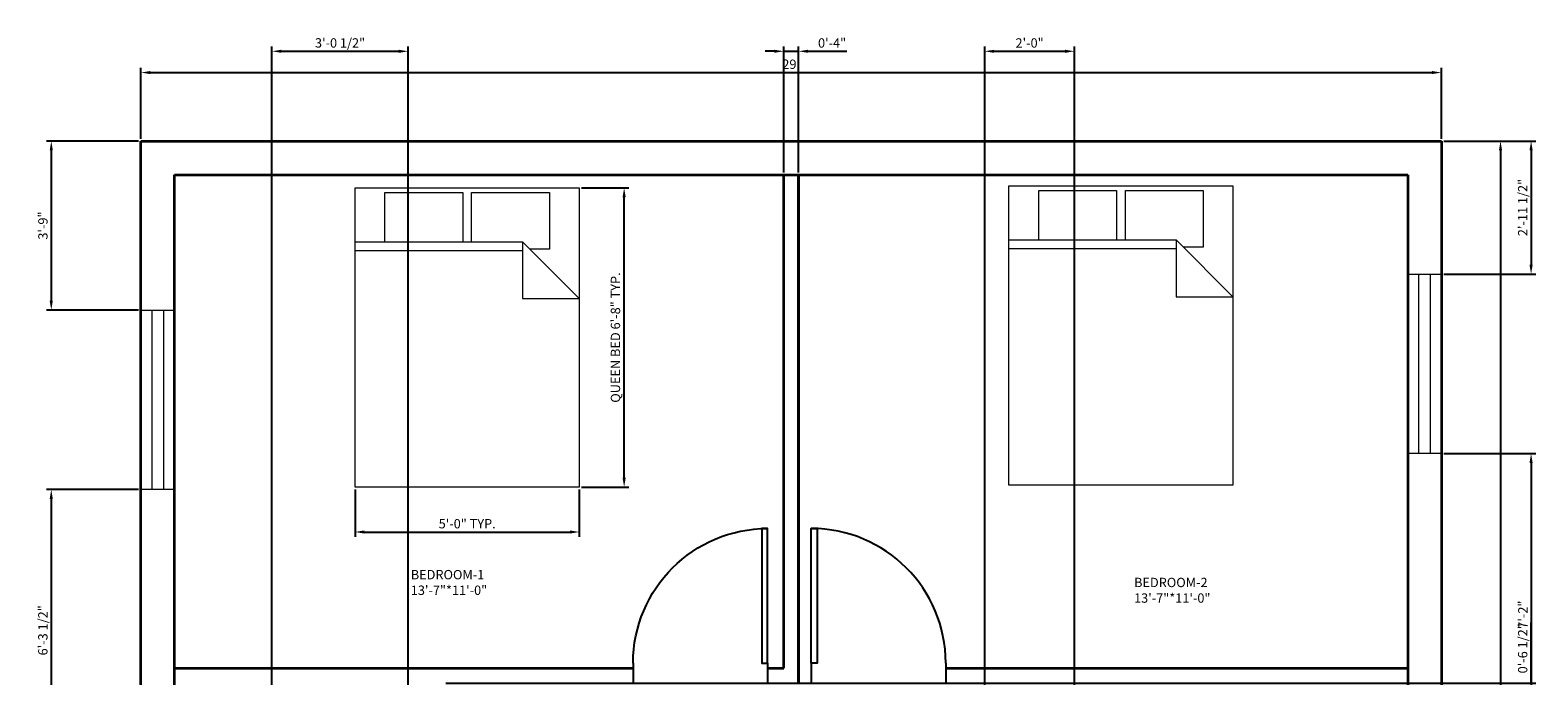
# Model space of a CAD drawing. Units: inches. Extents: x 2655 to 3059, y 1617 to 2098.
# Tile 3 of 3: x 2655 to 3059, y 1926 to 2098. Entities that reach past the tile are written whole.
import ezdxf

# ---------------------------------------------------------------- set-up
doc = ezdxf.new("R2010")
doc.units = ezdxf.units.IN
for name, color, linetype, lineweight in [('A-ANNO-DIMS', 2, 'Continuous', 18), ('A-AREA-IDEN', 7, 'Continuous', 18), ('A-DOOR', 3, 'Continuous', 25), ('A-FURN', 8, 'Continuous', 18), ('A-GLAZ', 4, 'Continuous', 18), ('A-WALL', 7, 'Continuous', 35)]:
    doc.layers.add(name, color=color, linetype=linetype, lineweight=lineweight)
doc.styles.get("Standard").update_dxf_attribs({"font": 'arial.ttf'})
doc.dimstyles.new('ISO-25', dxfattribs={"dimtxt": 2.5, "dimasz": 2.5, "dimexe": 1.25, "dimexo": 0.625, "dimtad": 1, "dimdec": 1, "dimlunit": 3, "dimtxsty": 'Standard', "dimcen": 2.5, "dimadec": 0, "dimazin": 0, "dimtfac": 1, "dimtdec": 1, "dimtmove": 0, "dimatfit": 3, "dimfxl": 1, "dimarcsym": 0})

# ---------------------------------------------------------------- blocks, each defined once
blk = doc.blocks.new('*U5')
for p, q in [((0, 0), (0, -6)), ((40, 0), (40, -6))]:
    blk.add_line(p, q)
blk.add_lwpolyline([(0, 0), (0, 40), (1.75, 40), (1.75, 0)], close=True)
blk.add_arc((0, 0), 40, 0, 90)
blk = doc.blocks.new('Bed - Queen')
for p, q in [((0, -80.00003), (0, 0)), ((0, 0), (59.99999, 0)), ((59.99999, 0), (59.99999, -80.00003)), ((7.99999, -1.2), (28.79998, -1.2)), ((7.99999, -14.4), (7.99999, -1.2)), ((28.79998, -1.2), (28.79998, -14.4)), ((31.19999, -1.2), (51.99999, -1.2)), ((31.19999, -14.4), (31.19999, -1.2)), ((51.99999, -1.2), (51.99999, -16.4)), ((0, -14.4), (44.8, -14.4)), ((59.99999, -29.6), (44.8, -14.4)), ((44.8, -14.4), (44.8, -29.6)), ((44.8, -16.8), (0, -16.8)), ((51.99999, -16.4), (46.79936, -16.4)), ((44.8, -29.6), (59.99999, -29.6)), ((59.99999, -80.00003), (0, -80.00003))]:
    blk.add_line(p, q)
blk = doc.blocks.new('*D9')
at = {"layer": 'A-ANNO-DIMS', "color": 0, "lineweight": -2, "transparency": 16777216}
for p, q in [((2684.77, 2069.39), (2684.77, 2088.33)), ((2687.27, 2087.08), (3030.27, 2087.08)), ((3032.77, 2069.39), (3032.77, 2088.33))]:
    blk.add_line(p, q, dxfattribs=at)
at = {"layer": 'A-ANNO-DIMS', "color": 0, "transparency": 16777216}
for points in [[(2687.27, 2087.5), (2687.27, 2086.66), (2684.77, 2087.08)], [(3030.27, 2087.5), (3030.27, 2086.66), (3032.77, 2087.08)]]:
    blk.add_solid(points, dxfattribs=at)
at = {"layer": 'Defpoints', "color": 0, "transparency": 16777216}
for p in [(3032.77, 2087.08), (2684.77, 2068.77), (3032.77, 2068.77)]:
    blk.add_point(p, dxfattribs=at)
at = {"layer": 'A-ANNO-DIMS', "color": 0, "transparency": 16777216, "insert": (2858.77, 2088.98), "char_height": 2.5, "attachment_point": 5}
blk.add_mtext("29'", dxfattribs=at)
blk = doc.blocks.new('*D10')
at = {"layer": 'A-ANNO-DIMS', "color": 0, "lineweight": -2, "transparency": 16777216}
for p, q in [((3033.39, 2068.77), (3049.84, 2068.77)), ((3048.59, 2066.27), (3048.59, 1651.27)), ((3033.39, 1648.77), (3049.84, 1648.77))]:
    blk.add_line(p, q, dxfattribs=at)
at = {"layer": 'A-ANNO-DIMS', "color": 0, "transparency": 16777216}
for points in [[(3048.17, 2066.27), (3049, 2066.27), (3048.59, 2068.77)], [(3048.17, 1651.27), (3049, 1651.27), (3048.59, 1648.77)]]:
    blk.add_solid(points, dxfattribs=at)
at = {"layer": 'Defpoints', "color": 0, "transparency": 16777216}
for p in [(3032.77, 2068.77), (3032.77, 1648.77), (3048.59, 1648.77)]:
    blk.add_point(p, dxfattribs=at)
at = {"layer": 'A-ANNO-DIMS', "color": 0, "transparency": 16777216, "insert": (3046.68, 1858.77), "char_height": 2.5, "attachment_point": 5, "rotation": 90}
blk.add_mtext("35'", dxfattribs=at)
blk = doc.blocks.new('WIN-48x9')
for p, q in [((0, 9), (48, 9)), ((0, 0), (0, 9)), ((48, 9), (48, 0)), ((0, 6), (48, 6)), ((48, 3), (0, 3)), ((48, 0), (0, 0))]:
    blk.add_line(p, q)
blk = doc.blocks.new('*D15')
at = {"layer": 'A-ANNO-DIMS', "color": 0, "lineweight": -2, "transparency": 16777216}
for p, q in [((2802.69, 2056.22), (2815.32, 2056.22)), ((2814.07, 1978.72), (2814.07, 2053.72)), ((2802.69, 1976.22), (2815.32, 1976.22))]:
    blk.add_line(p, q, dxfattribs=at)
at = {"layer": 'A-ANNO-DIMS', "color": 0, "transparency": 16777216}
for points in [[(2813.65, 2053.72), (2814.49, 2053.72), (2814.07, 2056.22)], [(2813.65, 1978.72), (2814.49, 1978.72), (2814.07, 1976.22)]]:
    blk.add_solid(points, dxfattribs=at)
at = {"layer": 'Defpoints', "color": 0, "transparency": 16777216}
for p in [(2802.07, 2056.22), (2814.07, 2056.22), (2802.07, 1976.22)]:
    blk.add_point(p, dxfattribs=at)
at = {"layer": 'A-ANNO-DIMS', "color": 0, "transparency": 16777216, "insert": (2812.07, 2016.22), "char_height": 2.5, "attachment_point": 5, "rotation": 90}
blk.add_mtext('QUEEN BED 6\'-8" TYP.', dxfattribs=at)
blk = doc.blocks.new('*D16')
at = {"layer": 'A-ANNO-DIMS', "color": 0, "lineweight": -2, "transparency": 16777216}
for p, q in [((2742.07, 1975.59), (2742.07, 1962.97)), ((2802.07, 1975.59), (2802.07, 1962.97)), ((2744.57, 1964.22), (2799.57, 1964.22))]:
    blk.add_line(p, q, dxfattribs=at)
at = {"layer": 'A-ANNO-DIMS', "color": 0, "transparency": 16777216}
for points in [[(2744.57, 1964.64), (2744.57, 1963.8), (2742.07, 1964.22)], [(2799.57, 1964.64), (2799.57, 1963.8), (2802.07, 1964.22)]]:
    blk.add_solid(points, dxfattribs=at)
at = {"layer": 'Defpoints', "color": 0, "transparency": 16777216}
for p in [(2742.07, 1976.22), (2802.07, 1976.22), (2802.07, 1964.22)]:
    blk.add_point(p, dxfattribs=at)
at = {"layer": 'A-ANNO-DIMS', "color": 0, "transparency": 16777216, "insert": (2772.07, 1966.12), "char_height": 2.5, "attachment_point": 5}
blk.add_mtext('5\'-0" TYP.', dxfattribs=at)
blk = doc.blocks.new('*D23')
at = {"layer": 'A-ANNO-DIMS', "color": 0, "lineweight": -2, "transparency": 16777216}
for p, q in [((2684.14, 2068.77), (2659.52, 2068.77)), ((2660.77, 2066.27), (2660.77, 2026.08)), ((2684.14, 2023.58), (2659.52, 2023.58))]:
    blk.add_line(p, q, dxfattribs=at)
at = {"layer": 'A-ANNO-DIMS', "color": 0, "transparency": 16777216}
for points in [[(2660.35, 2066.27), (2661.19, 2066.27), (2660.77, 2068.77)], [(2660.35, 2026.08), (2661.19, 2026.08), (2660.77, 2023.58)]]:
    blk.add_solid(points, dxfattribs=at)
at = {"layer": 'Defpoints', "color": 0, "transparency": 16777216}
for p in [(2684.77, 2068.77), (2660.77, 2023.58), (2684.77, 2023.58)]:
    blk.add_point(p, dxfattribs=at)
at = {"layer": 'A-ANNO-DIMS', "color": 0, "transparency": 16777216, "insert": (2658.87, 2046.17), "char_height": 2.5, "attachment_point": 5, "rotation": 90}
blk.add_mtext('3\'-9"', dxfattribs=at)
blk = doc.blocks.new('*D24')
at = {"layer": 'A-ANNO-DIMS', "color": 0, "lineweight": -2, "transparency": 16777216}
for p, q in [((2684.14, 1975.58), (2659.52, 1975.58)), ((2660.77, 1973.08), (2660.77, 1902.78)), ((2684.15, 1900.28), (2659.52, 1900.28))]:
    blk.add_line(p, q, dxfattribs=at)
at = {"layer": 'A-ANNO-DIMS', "color": 0, "transparency": 16777216}
for points in [[(2660.35, 1973.08), (2661.19, 1973.08), (2660.77, 1975.58)], [(2660.35, 1902.78), (2661.19, 1902.78), (2660.77, 1900.28)]]:
    blk.add_solid(points, dxfattribs=at)
at = {"layer": 'Defpoints', "color": 0, "transparency": 16777216}
for p in [(2684.77, 1975.58), (2660.77, 1900.28), (2684.78, 1900.28)]:
    blk.add_point(p, dxfattribs=at)
at = {"layer": 'A-ANNO-DIMS', "color": 0, "transparency": 16777216, "insert": (2658.85, 1937.93), "char_height": 2.5, "attachment_point": 5, "rotation": 90}
blk.add_mtext('6\'-3 1/2"', dxfattribs=at)
blk = doc.blocks.new('*D26')
at = {"layer": 'A-ANNO-DIMS', "color": 0, "lineweight": -2, "transparency": 16777216}
for p, q in [((3033.39, 2068.77), (3058.02, 2068.77)), ((3056.77, 2066.27), (3056.77, 2035.71)), ((3033.39, 2033.21), (3058.02, 2033.21))]:
    blk.add_line(p, q, dxfattribs=at)
at = {"layer": 'A-ANNO-DIMS', "color": 0, "transparency": 16777216}
for points in [[(3056.35, 2066.27), (3057.19, 2066.27), (3056.77, 2068.77)], [(3056.35, 2035.71), (3057.19, 2035.71), (3056.77, 2033.21)]]:
    blk.add_solid(points, dxfattribs=at)
at = {"layer": 'Defpoints', "color": 0, "transparency": 16777216}
for p in [(3032.77, 2068.77), (3032.77, 2033.21), (3056.77, 2033.21)]:
    blk.add_point(p, dxfattribs=at)
at = {"layer": 'A-ANNO-DIMS', "color": 0, "transparency": 16777216, "insert": (3054.85, 2050.99), "char_height": 2.5, "attachment_point": 5, "rotation": 90}
blk.add_mtext('2\'-11 1/2"', dxfattribs=at)
blk = doc.blocks.new('*D27')
at = {"layer": 'A-ANNO-DIMS', "color": 0, "lineweight": -2, "transparency": 16777216}
for p, q in [((3033.39, 1985.21), (3058.02, 1985.21)), ((3056.77, 1982.71), (3056.77, 1901.56)), ((3033.39, 1899.06), (3058.02, 1899.06))]:
    blk.add_line(p, q, dxfattribs=at)
at = {"layer": 'A-ANNO-DIMS', "color": 0, "transparency": 16777216}
for points in [[(3056.35, 1982.71), (3057.19, 1982.71), (3056.77, 1985.21)], [(3056.35, 1901.56), (3057.19, 1901.56), (3056.77, 1899.06)]]:
    blk.add_solid(points, dxfattribs=at)
at = {"layer": 'Defpoints', "color": 0, "transparency": 16777216}
for p in [(3032.77, 1985.21), (3032.77, 1899.06), (3056.77, 1899.06)]:
    blk.add_point(p, dxfattribs=at)
at = {"layer": 'A-ANNO-DIMS', "color": 0, "transparency": 16777216, "insert": (3054.89, 1942.13), "char_height": 2.5, "attachment_point": 5, "rotation": 90}
blk.add_mtext('7\'-2"', dxfattribs=at)
blk = doc.blocks.new('*D35')
at = {"layer": 'A-ANNO-DIMS', "color": 0, "lineweight": -2, "transparency": 16777216}
for p, q in [((2856.77, 2060.39), (2856.77, 2094.02)), ((2860.77, 2060.39), (2860.77, 2094.02)), ((2854.27, 2092.77), (2851.77, 2092.77)), ((2856.77, 2092.77), (2860.77, 2092.77)), ((2863.27, 2092.77), (2873.66, 2092.77))]:
    blk.add_line(p, q, dxfattribs=at)
at = {"layer": 'A-ANNO-DIMS', "color": 0, "transparency": 16777216}
for points in [[(2854.27, 2093.18), (2854.27, 2092.35), (2856.77, 2092.77)], [(2863.27, 2093.18), (2863.27, 2092.35), (2860.77, 2092.77)]]:
    blk.add_solid(points, dxfattribs=at)
at = {"layer": 'Defpoints', "color": 0, "transparency": 16777216}
for p in [(2860.77, 2092.77), (2856.77, 2059.77), (2860.77, 2059.77)]:
    blk.add_point(p, dxfattribs=at)
at = {"layer": 'A-ANNO-DIMS', "color": 0, "transparency": 16777216, "insert": (2869.72, 2094.67), "char_height": 2.5, "attachment_point": 5}
blk.add_mtext('0\'-4"', dxfattribs=at)
blk = doc.blocks.new('*D39')
at = {"layer": 'A-ANNO-DIMS', "color": 0, "lineweight": -2, "transparency": 16777216}
for p, q in [((2910.57, 1846.39), (2910.57, 2094.02)), ((2934.57, 1846.39), (2934.57, 2094.02)), ((2913.07, 2092.77), (2932.07, 2092.77))]:
    blk.add_line(p, q, dxfattribs=at)
at = {"layer": 'A-ANNO-DIMS', "color": 0, "transparency": 16777216}
for points in [[(2913.07, 2093.18), (2913.07, 2092.35), (2910.57, 2092.77)], [(2932.07, 2093.18), (2932.07, 2092.35), (2934.57, 2092.77)]]:
    blk.add_solid(points, dxfattribs=at)
at = {"layer": 'Defpoints', "color": 0, "transparency": 16777216}
for p in [(2934.57, 2092.77), (2910.57, 1845.77), (2934.57, 1845.77)]:
    blk.add_point(p, dxfattribs=at)
at = {"layer": 'A-ANNO-DIMS', "color": 0, "transparency": 16777216, "insert": (2922.57, 2094.67), "char_height": 2.5, "attachment_point": 5}
blk.add_mtext('2\'-0"', dxfattribs=at)
blk = doc.blocks.new('*D46')
at = {"layer": 'A-ANNO-DIMS', "color": 0, "lineweight": -2, "transparency": 16777216}
for p, q in [((2719.83, 1903.48), (2719.83, 2094.02)), ((2756.27, 1903.48), (2756.27, 2094.02)), ((2722.33, 2092.77), (2753.77, 2092.77))]:
    blk.add_line(p, q, dxfattribs=at)
at = {"layer": 'A-ANNO-DIMS', "color": 0, "transparency": 16777216}
for points in [[(2722.33, 2093.18), (2722.33, 2092.35), (2719.83, 2092.77)], [(2753.77, 2093.18), (2753.77, 2092.35), (2756.27, 2092.77)]]:
    blk.add_solid(points, dxfattribs=at)
at = {"layer": 'Defpoints', "color": 0, "transparency": 16777216}
for p in [(2756.27, 2092.77), (2719.83, 1902.86), (2756.27, 1902.86)]:
    blk.add_point(p, dxfattribs=at)
at = {"layer": 'A-ANNO-DIMS', "color": 0, "transparency": 16777216, "insert": (2738.05, 2094.68), "char_height": 2.5, "attachment_point": 5}
blk.add_mtext('3\'-0 1/2"', dxfattribs=at)
blk = doc.blocks.new('*D50')
at = {"layer": 'A-ANNO-DIMS', "color": 0, "lineweight": -2, "transparency": 16777216}
for p, q in [((3056.77, 1923.77), (3056.77, 1939.99)), ((2766.39, 1923.77), (3058.02, 1923.77)), ((3056.77, 1919.87), (3056.77, 1921.27)), ((2751.1, 1917.37), (3058.02, 1917.37))]:
    blk.add_line(p, q, dxfattribs=at)
at = {"layer": 'A-ANNO-DIMS', "color": 0, "transparency": 16777216}
for points in [[(3056.35, 1921.27), (3057.19, 1921.27), (3056.77, 1923.77)], [(3056.35, 1919.87), (3057.19, 1919.87), (3056.77, 1917.37)]]:
    blk.add_solid(points, dxfattribs=at)
at = {"layer": 'Defpoints', "color": 0, "transparency": 16777216}
for p in [(2765.77, 1923.77), (3056.77, 1923.77), (2750.48, 1917.37)]:
    blk.add_point(p, dxfattribs=at)
at = {"layer": 'A-ANNO-DIMS', "color": 0, "transparency": 16777216, "insert": (3054.85, 1933.13), "char_height": 2.5, "attachment_point": 5, "rotation": 90}
blk.add_mtext('0\'-6 1/2"', dxfattribs=at)

msp = doc.modelspace()

# ---------------------------------------------------------------- linework, layer by layer
at = {"layer": 'A-WALL'}
for p, q in [((2684.77, 2068.77), (3032.77, 2068.77)), ((2684.77, 1648.77), (2684.77, 2068.77)), ((3032.77, 2068.77), (3032.77, 1648.77)), ((2693.77, 2059.77), (3023.77, 2059.77)), ((2693.77, 1754.27), (2693.77, 2059.77)), ((2856.77, 1927.77), (2856.77, 2059.77)), ((2860.77, 2059.77), (2860.77, 1923.77)), ((2860.77, 1923.77), (2860.77, 2059.77)), ((3023.77, 2059.77), (3023.77, 1657.77)), ((2693.77, 1927.77), (2816.47, 1927.77)), ((2852.47, 1927.77), (2856.77, 1927.77)), ((2900.13, 1927.77), (3023.77, 1927.77))]:
    msp.add_line(p, q, dxfattribs=at)

# ---------------------------------------------------------------- block references
at = {"layer": 'A-DOOR', "yscale": 0.9, "zscale": 0.9}
for p, xscale in [((2852.47, 1929.17), -0.9), ((2864.13, 1929.17), 0.9)]:
    msp.add_blockref('*U5', p, dxfattribs=dict(at, xscale=xscale))
at = {"layer": 'A-FURN'}
for p in [(2742.07, 2056.22), (2917, 2056.75)]:
    msp.add_blockref('Bed - Queen', p, dxfattribs=at)
at = {"layer": 'A-GLAZ'}
for p, rotation in [((3032.77, 1985.21), 90.00000000000095), ((2693.77, 1975.58), 90.00000000000115)]:
    msp.add_blockref('WIN-48x9', p, dxfattribs=dict(at, rotation=rotation))

# ---------------------------------------------------------------- texts
at = {"layer": 'A-AREA-IDEN', "char_height": 2.5, "attachment_point": 1}
for s, width, insert in [('BEDROOM-1\\P13\'-7"*11\'-0"', 68.1375, (2756.98, 1954.07)), ('BEDROOM-2\\P13\'-7"*11\'-0"', 48.8552, (2950.53, 1951.98))]:
    msp.add_mtext_dynamic_manual_height_columns(s, width=width, gutter_width=12.5, heights=[0], dxfattribs=dict(at, insert=insert))

# ---------------------------------------------------------------- dimensions: what is measured, and where the dimension line sits
at = {"layer": 'A-ANNO-DIMS'}
for base, p1, p2, override, picture, middle in [((2756.27, 2092.77), (2719.83, 1902.86), (2756.27, 1902.86), {"dimdec": 1, "dimlfac": 1, "dimrnd": 0, "dimzin": 1, "dimdsep": 46, "dimlunit": 4, "dimfrac": 2}, '*D46', (2738.05, 2094.68)), ((2860.77, 2092.77), (2856.77, 2059.77), (2860.77, 2059.77), {"dimdec": 1, "dimlfac": 1, "dimrnd": 0, "dimzin": 1, "dimdsep": 46, "dimlunit": 4, "dimfrac": 2}, '*D35', (2869.72, 2094.67)), ((2934.57, 2092.77), (2910.57, 1845.77), (2934.57, 1845.77), {"dimdec": 1, "dimlfac": 1, "dimrnd": 0, "dimzin": 1, "dimdsep": 46, "dimlunit": 4, "dimfrac": 2}, '*D39', (2922.57, 2094.67)), ((3032.77, 2087.08), (2684.77, 2068.77), (3032.77, 2068.77), {"dimclrd": 0, "dimclre": 0, "dimclrt": 0}, '*D9', (2858.77, 2088.98))]:
    dim = msp.add_linear_dim(base=base, p1=p1, p2=p2, dimstyle='ISO-25', override=override, dxfattribs=at)
    dim.commit()
    dim.dimension.update_dxf_attribs({"geometry": picture, "text_midpoint": middle})
for base, p1, p2, override, picture, middle in [((2660.77, 2023.58), (2684.77, 2068.77), (2684.77, 2023.58), {"dimdec": 1, "dimlfac": 1, "dimrnd": 0, "dimzin": 1, "dimdsep": 46, "dimlunit": 4, "dimfrac": 2}, '*D23', (2658.87, 2046.17)), ((3048.59, 1648.77), (3032.77, 2068.77), (3032.77, 1648.77), {"dimclrd": 0, "dimclre": 0, "dimclrt": 0}, '*D10', (3046.68, 1858.77)), ((3056.77, 2033.21), (3032.77, 2068.77), (3032.77, 2033.21), {"dimdec": 1, "dimlfac": 1, "dimrnd": 0, "dimzin": 1, "dimdsep": 46, "dimlunit": 4, "dimfrac": 2}, '*D26', (3054.85, 2050.99)), ((3056.7686, 1899.0573), (3032.7686, 1985.2098), (3032.7677, 1899.0573), {"dimdec": 1, "dimlfac": 1, "dimrnd": 0, "dimzin": 1, "dimdsep": 46, "dimlunit": 4, "dimfrac": 2}, '*D27', (3054.8885, 1942.1335)), ((2660.77, 1900.28), (2684.77, 1975.58), (2684.78, 1900.28), {"dimdec": 1, "dimlfac": 1, "dimrnd": 0, "dimzin": 1, "dimdsep": 46, "dimlunit": 4, "dimfrac": 2}, '*D24', (2658.85, 1937.93)), ((3056.77, 1923.77), (2750.48, 1917.37), (2765.77, 1923.77), {"dimdec": 1, "dimlfac": 1, "dimrnd": 0, "dimzin": 1, "dimdsep": 46, "dimlunit": 4, "dimfrac": 2}, '*D50', (3054.85, 1933.13))]:
    dim = msp.add_linear_dim(base=base, p1=p1, p2=p2, angle=90, dimstyle='ISO-25', override=override, dxfattribs=at)
    dim.commit()
    dim.dimension.update_dxf_attribs({"geometry": picture, "text_midpoint": middle})
dim = msp.add_linear_dim(base=(2814.07, 2056.22), p1=(2802.07, 1976.22), p2=(2802.07, 2056.22), angle=90, text='QUEEN BED <> TYP.', dimstyle='ISO-25', override={"dimdec": 1, "dimlfac": 1, "dimrnd": 0, "dimzin": 1, "dimdsep": 46, "dimlunit": 4, "dimfrac": 2}, dxfattribs=at)
dim.commit()
dim.dimension.update_dxf_attribs({"geometry": '*D15', "text_midpoint": (2812.07, 2016.22)})
dim = msp.add_linear_dim(base=(2802.07, 1964.22), p1=(2742.07, 1976.22), p2=(2802.07, 1976.22), text='<> TYP.', dimstyle='ISO-25', override={"dimdec": 1, "dimlfac": 1, "dimrnd": 0, "dimzin": 1, "dimdsep": 46, "dimlunit": 4, "dimfrac": 2}, dxfattribs=at)
dim.commit()
dim.dimension.update_dxf_attribs({"geometry": '*D16', "text_midpoint": (2772.07, 1966.12)})

doc.saveas('drawing.dxf')
